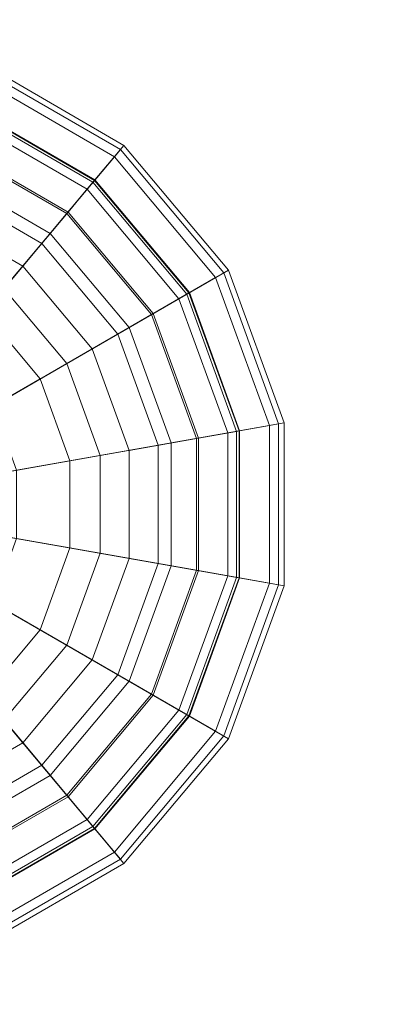
# Model space of a CAD drawing. Units: inches. Extents: x 375 to 1122, y 27 to 1069.
# Tile 93 of 155: x 730.25 to 731.282, y 859.033 to 861.878. Entities that reach past the tile are written whole.
import ezdxf

# ---------------------------------------------------------------- set-up
doc = ezdxf.new("R2010")
doc.units = ezdxf.units.IN
doc.layers.add('A-ANNO-DIMS', color=2, linetype='Continuous', lineweight=18)
doc.layers.add('Furniture', color=30, linetype='Continuous', lineweight=18)
doc.styles.get("Standard").update_dxf_attribs({"font": 'arial.ttf'})
doc.dimstyles.new('ISO-25', dxfattribs={"dimtxt": 12, "dimasz": 2.5, "dimexe": 1.5, "dimexo": 1.5, "dimtad": 1, "dimdec": 1, "dimlunit": 3, "dimtxsty": 'Standard', "dimblk": 'ARCHTICK', "dimcen": 2.5, "dimadec": 0, "dimazin": 0, "dimtfac": 1, "dimtdec": 1, "dimtmove": 0, "dimatfit": 3, "dimfxl": 1.5, "dimfxlon": 1, "dimarcsym": 0})

# ---------------------------------------------------------------- blocks, each defined once
blk = doc.blocks.new('A$C403C54AD')
for points in [[(1.940462, 1.15174, -0.060915), (1.946342, 1.118392, -0.057836), (1.946342, 1.118392, -0.057836), (1.929411, 1.147718, -0.060915)], [(1.941029, 1.148524, -0.057684), (1.940462, 1.15174, -0.060915), (1.929411, 1.147718, -0.060915), (1.931044, 1.144889, -0.057684)], [(1.941036, 1.148484, 0.102069), (1.940532, 1.151347, 0.088845), (1.929611, 1.147372, 0.088845), (1.931064, 1.144854, 0.102069)], [(1.940532, 1.151347, 0.088845), (1.940649, 1.150682, 0.060603), (1.929948, 1.146788, 0.060603), (1.929611, 1.147372, 0.088845)], [(1.952223, 1.15174, -0.060915), (1.946342, 1.118392, -0.057836), (1.946342, 1.118392, -0.057836), (1.940462, 1.15174, -0.060915)], [(1.951655, 1.148524, -0.057684), (1.952223, 1.15174, -0.060915), (1.940462, 1.15174, -0.060915), (1.941029, 1.148524, -0.057684)], [(1.951648, 1.148484, 0.102069), (1.952153, 1.151347, 0.088845), (1.940532, 1.151347, 0.088845), (1.941036, 1.148484, 0.102069)], [(1.952153, 1.151347, 0.088845), (1.952036, 1.150682, 0.060603), (1.940649, 1.150682, 0.060603), (1.940532, 1.151347, 0.088845)], [(1.963274, 1.147718, -0.060915), (1.946342, 1.118392, -0.057836), (1.946342, 1.118392, -0.057836), (1.952223, 1.15174, -0.060915)], [(1.96162, 1.144854, 0.102069), (1.963074, 1.147372, 0.088845), (1.952153, 1.151347, 0.088845), (1.951648, 1.148484, 0.102069)], [(1.961641, 1.144889, -0.057684), (1.963274, 1.147718, -0.060915), (1.952223, 1.15174, -0.060915), (1.951655, 1.148524, -0.057684)], [(1.963074, 1.147372, 0.088845), (1.962737, 1.146788, 0.060603), (1.952036, 1.150682, 0.060603), (1.952153, 1.151347, 0.088845)], [(1.940649, 1.150682, 0.060603), (1.94158, 1.145399, 0.042594), (1.932631, 1.142142, 0.042594), (1.929948, 1.146788, 0.060603)], [(1.952036, 1.150682, 0.060603), (1.951105, 1.145399, 0.042594), (1.94158, 1.145399, 0.042594), (1.940649, 1.150682, 0.060603)], [(1.962737, 1.146788, 0.060603), (1.960054, 1.142142, 0.042594), (1.951105, 1.145399, 0.042594), (1.952036, 1.150682, 0.060603)], [(1.943874, 1.13239, -0.054409), (1.941029, 1.148524, -0.057684), (1.931044, 1.144889, -0.057684), (1.939235, 1.130702, -0.054409)], [(1.941904, 1.143563, 0.111475), (1.941036, 1.148484, 0.102069), (1.931064, 1.144854, 0.102069), (1.933563, 1.140527, 0.111475)], [(1.941067, 1.148309, 0.088628), (1.941555, 1.145542, 0.101264), (1.932558, 1.142268, 0.101264), (1.931153, 1.144701, 0.088628)], [(1.941182, 1.147661, 0.061088), (1.941067, 1.148309, 0.088628), (1.931153, 1.144701, 0.088628), (1.931482, 1.144131, 0.061088)], [(1.948811, 1.13239, -0.054409), (1.951655, 1.148524, -0.057684), (1.941029, 1.148524, -0.057684), (1.943874, 1.13239, -0.054409)], [(1.950781, 1.143563, 0.111475), (1.951648, 1.148484, 0.102069), (1.941036, 1.148484, 0.102069), (1.941904, 1.143563, 0.111475)], [(1.951618, 1.148309, 0.088628), (1.95113, 1.145542, 0.101264), (1.941555, 1.145542, 0.101264), (1.941067, 1.148309, 0.088628)], [(1.951503, 1.147661, 0.061088), (1.951618, 1.148309, 0.088628), (1.941067, 1.148309, 0.088628), (1.941182, 1.147661, 0.061088)], [(1.95345, 1.130702, -0.054409), (1.961641, 1.144889, -0.057684), (1.951655, 1.148524, -0.057684), (1.948811, 1.13239, -0.054409)], [(1.959122, 1.140527, 0.111475), (1.96162, 1.144854, 0.102069), (1.951648, 1.148484, 0.102069), (1.950781, 1.143563, 0.111475)], [(1.961532, 1.144701, 0.088628), (1.960127, 1.142268, 0.101264), (1.95113, 1.145542, 0.101264), (1.951618, 1.148309, 0.088628)], [(1.961203, 1.144131, 0.061088), (1.961532, 1.144701, 0.088628), (1.951618, 1.148309, 0.088628), (1.951503, 1.147661, 0.061088)], [(1.929411, 1.147718, -0.060915), (1.946342, 1.118392, -0.057836), (1.946342, 1.118392, -0.057836), (1.920403, 1.140158, -0.060915)], [(1.931044, 1.144889, -0.057684), (1.929411, 1.147718, -0.060915), (1.920403, 1.140158, -0.060915), (1.922904, 1.138059, -0.057684)], [(1.942068, 1.142631, 0.043942), (1.941182, 1.147661, 0.061088), (1.931482, 1.144131, 0.061088), (1.934036, 1.139708, 0.043942)], [(1.950616, 1.142631, 0.043942), (1.951503, 1.147661, 0.061088), (1.941182, 1.147661, 0.061088), (1.942068, 1.142631, 0.043942)], [(1.972282, 1.140158, -0.060915), (1.946342, 1.118392, -0.057836), (1.946342, 1.118392, -0.057836), (1.963274, 1.147718, -0.060915)], [(1.958649, 1.139708, 0.043942), (1.961203, 1.144131, 0.061088), (1.951503, 1.147661, 0.061088), (1.950616, 1.142631, 0.043942)], [(1.969781, 1.138059, -0.057684), (1.972282, 1.140158, -0.060915), (1.963274, 1.147718, -0.060915), (1.961641, 1.144889, -0.057684)], [(1.931064, 1.144854, 0.102069), (1.929611, 1.147372, 0.088845), (1.920708, 1.139902, 0.088845), (1.922935, 1.138033, 0.102069)], [(1.929611, 1.147372, 0.088845), (1.929948, 1.146788, 0.060603), (1.921225, 1.139468, 0.060603), (1.920708, 1.139902, 0.088845)], [(1.96975, 1.138033, 0.102069), (1.971977, 1.139902, 0.088845), (1.963074, 1.147372, 0.088845), (1.96162, 1.144854, 0.102069)], [(1.971977, 1.139902, 0.088845), (1.97146, 1.139468, 0.060603), (1.962737, 1.146788, 0.060603), (1.963074, 1.147372, 0.088845)], [(1.929948, 1.146788, 0.060603), (1.932631, 1.142142, 0.042594), (1.925335, 1.13602, 0.042594), (1.921225, 1.139468, 0.060603)], [(1.97146, 1.139468, 0.060603), (1.96735, 1.13602, 0.042594), (1.960054, 1.142142, 0.042594), (1.962737, 1.146788, 0.060603)], [(1.941555, 1.145542, 0.101264), (1.942439, 1.140532, 0.111475), (1.935102, 1.137861, 0.111475), (1.932558, 1.142268, 0.101264)], [(1.94158, 1.145399, 0.042594), (1.942807, 1.13844, 0.032362), (1.936164, 1.136022, 0.032362), (1.932631, 1.142142, 0.042594)], [(1.95113, 1.145542, 0.101264), (1.950246, 1.140532, 0.111475), (1.942439, 1.140532, 0.111475), (1.941555, 1.145542, 0.101264)], [(1.951105, 1.145399, 0.042594), (1.949878, 1.13844, 0.032362), (1.942807, 1.13844, 0.032362), (1.94158, 1.145399, 0.042594)], [(1.960054, 1.142142, 0.042594), (1.956521, 1.136022, 0.032362), (1.949878, 1.13844, 0.032362), (1.951105, 1.145399, 0.042594)], [(1.960127, 1.142268, 0.101264), (1.957583, 1.137861, 0.111475), (1.950246, 1.140532, 0.111475), (1.95113, 1.145542, 0.101264)], [(1.939235, 1.130702, -0.054409), (1.931044, 1.144889, -0.057684), (1.922904, 1.138059, -0.057684), (1.935454, 1.127529, -0.054409)], [(1.933563, 1.140527, 0.111475), (1.931064, 1.144854, 0.102069), (1.922935, 1.138033, 0.102069), (1.926763, 1.134821, 0.111475)], [(1.931153, 1.144701, 0.088628), (1.932558, 1.142268, 0.101264), (1.925223, 1.136113, 0.101264), (1.923071, 1.137919, 0.088628)], [(1.931482, 1.144131, 0.061088), (1.931153, 1.144701, 0.088628), (1.923071, 1.137919, 0.088628), (1.923575, 1.137496, 0.061088)], [(1.957231, 1.127529, -0.054409), (1.969781, 1.138059, -0.057684), (1.961641, 1.144889, -0.057684), (1.95345, 1.130702, -0.054409)], [(1.965922, 1.134821, 0.111475), (1.96975, 1.138033, 0.102069), (1.96162, 1.144854, 0.102069), (1.959122, 1.140527, 0.111475)], [(1.969614, 1.137919, 0.088628), (1.967462, 1.136113, 0.101264), (1.960127, 1.142268, 0.101264), (1.961532, 1.144701, 0.088628)], [(1.96911, 1.137496, 0.061088), (1.969614, 1.137919, 0.088628), (1.961532, 1.144701, 0.088628), (1.961203, 1.144131, 0.061088)], [(1.934036, 1.139708, 0.043942), (1.931482, 1.144131, 0.061088), (1.923575, 1.137496, 0.061088), (1.927488, 1.134213, 0.043942)], [(1.965197, 1.134213, 0.043942), (1.96911, 1.137496, 0.061088), (1.961203, 1.144131, 0.061088), (1.958649, 1.139708, 0.043942)], [(1.942439, 1.140532, 0.111475), (1.941904, 1.143563, 0.111475), (1.933563, 1.140527, 0.111475), (1.935102, 1.137861, 0.111475)], [(1.950246, 1.140532, 0.111475), (1.950781, 1.143563, 0.111475), (1.941904, 1.143563, 0.111475), (1.942439, 1.140532, 0.111475)], [(1.957583, 1.137861, 0.111475), (1.959122, 1.140527, 0.111475), (1.950781, 1.143563, 0.111475), (1.950246, 1.140532, 0.111475)], [(1.943195, 1.136244, 0.03455), (1.942068, 1.142631, 0.043942), (1.934036, 1.139708, 0.043942), (1.937279, 1.134091, 0.03455)], [(1.94949, 1.136244, 0.03455), (1.950616, 1.142631, 0.043942), (1.942068, 1.142631, 0.043942), (1.943195, 1.136244, 0.03455)], [(1.955406, 1.134091, 0.03455), (1.958649, 1.139708, 0.043942), (1.950616, 1.142631, 0.043942), (1.94949, 1.136244, 0.03455)], [(1.932558, 1.142268, 0.101264), (1.935102, 1.137861, 0.111475), (1.929121, 1.132843, 0.111475), (1.925223, 1.136113, 0.101264)], [(1.932631, 1.142142, 0.042594), (1.936164, 1.136022, 0.032362), (1.930748, 1.131478, 0.032362), (1.925335, 1.13602, 0.042594)], [(1.96735, 1.13602, 0.042594), (1.961937, 1.131478, 0.032362), (1.956521, 1.136022, 0.032362), (1.960054, 1.142142, 0.042594)], [(1.967462, 1.136113, 0.101264), (1.963564, 1.132843, 0.111475), (1.957583, 1.137861, 0.111475), (1.960127, 1.142268, 0.101264)], [(1.935102, 1.137861, 0.111475), (1.933563, 1.140527, 0.111475), (1.926763, 1.134821, 0.111475), (1.929121, 1.132843, 0.111475)], [(1.963564, 1.132843, 0.111475), (1.965922, 1.134821, 0.111475), (1.959122, 1.140527, 0.111475), (1.957583, 1.137861, 0.111475)], [(1.920403, 1.140158, -0.060915), (1.946342, 1.118392, -0.057836), (1.946342, 1.118392, -0.057836), (1.914522, 1.129974, -0.060915)], [(1.922904, 1.138059, -0.057684), (1.920403, 1.140158, -0.060915), (1.914522, 1.129974, -0.060915), (1.917591, 1.128857, -0.057684)], [(1.922935, 1.138033, 0.102069), (1.920708, 1.139902, 0.088845), (1.914897, 1.129837, 0.088845), (1.917629, 1.128843, 0.102069)], [(1.920708, 1.139902, 0.088845), (1.921225, 1.139468, 0.060603), (1.915531, 1.129606, 0.060603), (1.914897, 1.129837, 0.088845)], [(1.937279, 1.134091, 0.03455), (1.934036, 1.139708, 0.043942), (1.927488, 1.134213, 0.043942), (1.932456, 1.130044, 0.03455)], [(1.978163, 1.129974, -0.060915), (1.946342, 1.118392, -0.057836), (1.946342, 1.118392, -0.057836), (1.972282, 1.140158, -0.060915)], [(1.960229, 1.130044, 0.03455), (1.965197, 1.134213, 0.043942), (1.958649, 1.139708, 0.043942), (1.955406, 1.134091, 0.03455)], [(1.975056, 1.128843, 0.102069), (1.977788, 1.129837, 0.088845), (1.971977, 1.139902, 0.088845), (1.96975, 1.138033, 0.102069)], [(1.975094, 1.128857, -0.057684), (1.978163, 1.129974, -0.060915), (1.972282, 1.140158, -0.060915), (1.969781, 1.138059, -0.057684)], [(1.977788, 1.129837, 0.088845), (1.977153, 1.129606, 0.060603), (1.97146, 1.139468, 0.060603), (1.971977, 1.139902, 0.088845)], [(1.921225, 1.139468, 0.060603), (1.925335, 1.13602, 0.042594), (1.920572, 1.127772, 0.042594), (1.915531, 1.129606, 0.060603)], [(1.977153, 1.129606, 0.060603), (1.972112, 1.127772, 0.042594), (1.96735, 1.13602, 0.042594), (1.97146, 1.139468, 0.060603)], [(1.942807, 1.13844, 0.032362), (1.944585, 1.128357, 0.024995), (1.941283, 1.127155, 0.024995), (1.936164, 1.136022, 0.032362)], [(1.949878, 1.13844, 0.032362), (1.9481, 1.128357, 0.024995), (1.944585, 1.128357, 0.024995), (1.942807, 1.13844, 0.032362)], [(1.956521, 1.136022, 0.032362), (1.951402, 1.127155, 0.024995), (1.9481, 1.128357, 0.024995), (1.949878, 1.13844, 0.032362)], [(1.935454, 1.127529, -0.054409), (1.922904, 1.138059, -0.057684), (1.917591, 1.128857, -0.057684), (1.932985, 1.123254, -0.054409)], [(1.926763, 1.134821, 0.111475), (1.922935, 1.138033, 0.102069), (1.917629, 1.128843, 0.102069), (1.922324, 1.127134, 0.111475)], [(1.923071, 1.137919, 0.088628), (1.925223, 1.136113, 0.101264), (1.920436, 1.127821, 0.101264), (1.917796, 1.128782, 0.088628)], [(1.923575, 1.137496, 0.061088), (1.923071, 1.137919, 0.088628), (1.917796, 1.128782, 0.088628), (1.918414, 1.128557, 0.061088)], [(1.9597, 1.123254, -0.054409), (1.975094, 1.128857, -0.057684), (1.969781, 1.138059, -0.057684), (1.957231, 1.127529, -0.054409)], [(1.970361, 1.127134, 0.111475), (1.975056, 1.128843, 0.102069), (1.96975, 1.138033, 0.102069), (1.965922, 1.134821, 0.111475)], [(1.974889, 1.128782, 0.088628), (1.972249, 1.127821, 0.101264), (1.967462, 1.136113, 0.101264), (1.969614, 1.137919, 0.088628)], [(1.974271, 1.128557, 0.061088), (1.974889, 1.128782, 0.088628), (1.969614, 1.137919, 0.088628), (1.96911, 1.137496, 0.061088)], [(1.927488, 1.134213, 0.043942), (1.923575, 1.137496, 0.061088), (1.918414, 1.128557, 0.061088), (1.923214, 1.12681, 0.043942)], [(1.969471, 1.12681, 0.043942), (1.974271, 1.128557, 0.061088), (1.96911, 1.137496, 0.061088), (1.965197, 1.134213, 0.043942)], [(1.944796, 1.127161, 0.027913), (1.943195, 1.136244, 0.03455), (1.937279, 1.134091, 0.03455), (1.94189, 1.126103, 0.027913)], [(1.947889, 1.127161, 0.027913), (1.94949, 1.136244, 0.03455), (1.943195, 1.136244, 0.03455), (1.944796, 1.127161, 0.027913)], [(1.950795, 1.126103, 0.027913), (1.955406, 1.134091, 0.03455), (1.94949, 1.136244, 0.03455), (1.947889, 1.127161, 0.027913)], [(1.925223, 1.136113, 0.101264), (1.929121, 1.132843, 0.111475), (1.925217, 1.126081, 0.111475), (1.920436, 1.127821, 0.101264)], [(1.925335, 1.13602, 0.042594), (1.930748, 1.131478, 0.032362), (1.927213, 1.125355, 0.032362), (1.920572, 1.127772, 0.042594)], [(1.936164, 1.136022, 0.032362), (1.941283, 1.127155, 0.024995), (1.938591, 1.124896, 0.024995), (1.930748, 1.131478, 0.032362)], [(1.961937, 1.131478, 0.032362), (1.954094, 1.124896, 0.024995), (1.951402, 1.127155, 0.024995), (1.956521, 1.136022, 0.032362)], [(1.972112, 1.127772, 0.042594), (1.965472, 1.125355, 0.032362), (1.961937, 1.131478, 0.032362), (1.96735, 1.13602, 0.042594)], [(1.972249, 1.127821, 0.101264), (1.967468, 1.126081, 0.111475), (1.963564, 1.132843, 0.111475), (1.967462, 1.136113, 0.101264)], [(1.929121, 1.132843, 0.111475), (1.926763, 1.134821, 0.111475), (1.922324, 1.127134, 0.111475), (1.925217, 1.126081, 0.111475)], [(1.967468, 1.126081, 0.111475), (1.970361, 1.127134, 0.111475), (1.965922, 1.134821, 0.111475), (1.963564, 1.132843, 0.111475)], [(1.932456, 1.130044, 0.03455), (1.927488, 1.134213, 0.043942), (1.923214, 1.12681, 0.043942), (1.929308, 1.124592, 0.03455)], [(1.94189, 1.126103, 0.027913), (1.937279, 1.134091, 0.03455), (1.932456, 1.130044, 0.03455), (1.939522, 1.124116, 0.027913)], [(1.953163, 1.124116, 0.027913), (1.960229, 1.130044, 0.03455), (1.955406, 1.134091, 0.03455), (1.950795, 1.126103, 0.027913)], [(1.963376, 1.124592, 0.03455), (1.969471, 1.12681, 0.043942), (1.965197, 1.134213, 0.043942), (1.960229, 1.130044, 0.03455)]]:
    blk.add_3dface(points)
blk = doc.blocks.new('_ArchTick')
at = {"color": 0, "linetype": 'ByBlock', "const_width": 0.15}
blk.add_lwpolyline([(-0.5, -0.5), (0.5, 0.5)], dxfattribs=at)
blk = doc.blocks.new('*D85')
at = {"layer": 'A-ANNO-DIMS', "color": 0, "lineweight": -2, "transparency": 16777216}
for p, q in [((401.5073, 868.5277), (398.5073, 868.5277)), ((400.0073, 814.5277), (400.0073, 868.5277)), ((401.5073, 814.5277), (398.5073, 814.5277))]:
    blk.add_line(p, q, dxfattribs=at)
at = {"layer": 'Defpoints', "color": 0, "transparency": 16777216}
for p in [(400.0073, 868.5277), (845.0073, 868.5277), (845.0073, 814.5277)]:
    blk.add_point(p, dxfattribs=at)
at = {"layer": 'A-ANNO-DIMS', "color": 0, "lineweight": -2, "transparency": 16777216, "xscale": 2.5, "yscale": 2.5, "zscale": 2.5}
for p, rotation in [((400.0073, 868.5277), 90), ((400.0073, 814.5277), 270)]:
    blk.add_blockref('_ArchTick', p, dxfattribs=dict(at, rotation=rotation))
at = {"layer": 'A-ANNO-DIMS', "color": 0, "transparency": 16777216, "insert": (393.2555, 841.5277), "char_height": 12, "attachment_point": 5, "rotation": 90}
blk.add_mtext('4\'-6"', dxfattribs=at)
blk = doc.blocks.new('*D88')
at = {"layer": 'A-ANNO-DIMS', "color": 0, "lineweight": -2, "transparency": 16777216}
for p, q in [((731.0073, 1052.5277), (731.0073, 1055.5277)), ((854.0073, 1052.5277), (854.0073, 1055.5277)), ((731.0073, 1054.0277), (854.0073, 1054.0277))]:
    blk.add_line(p, q, dxfattribs=at)
at = {"layer": 'Defpoints', "color": 0, "transparency": 16777216}
for p in [(854.0073, 1054.0277), (731.0073, 502.5277), (854.0073, 502.5277)]:
    blk.add_point(p, dxfattribs=at)
at = {"layer": 'A-ANNO-DIMS', "color": 0, "lineweight": -2, "transparency": 16777216, "xscale": 2.5, "yscale": 2.5, "zscale": 2.5, "rotation": 180}
blk.add_blockref('_ArchTick', (731.0073, 1054.0277), dxfattribs=at)
at = {"layer": 'A-ANNO-DIMS', "color": 0, "lineweight": -2, "transparency": 16777216, "xscale": 2.5, "yscale": 2.5, "zscale": 2.5}
blk.add_blockref('_ArchTick', (854.0073, 1054.0277), dxfattribs=at)
at = {"layer": 'A-ANNO-DIMS', "color": 0, "transparency": 16777216, "insert": (792.5073, 1060.7837), "char_height": 12, "attachment_point": 5}
blk.add_mtext('10\'-3"', dxfattribs=at)
blk = doc.blocks.new('*D91')
at = {"layer": 'A-ANNO-DIMS', "color": 0, "lineweight": -2, "transparency": 16777216}
for p, q in [((728.0073, 1052.5277), (728.0073, 1055.5277)), ((788.0073, 1052.5277), (788.0073, 1055.5277)), ((728.0073, 1054.0277), (788.0073, 1054.0277))]:
    blk.add_line(p, q, dxfattribs=at)
at = {"layer": 'Defpoints', "color": 0, "transparency": 16777216}
for p in [(788.0073, 1054.0277), (728.0073, 774.0277), (788.0073, 774.0277)]:
    blk.add_point(p, dxfattribs=at)
at = {"layer": 'A-ANNO-DIMS', "color": 0, "lineweight": -2, "transparency": 16777216, "xscale": 2.5, "yscale": 2.5, "zscale": 2.5, "rotation": 180}
blk.add_blockref('_ArchTick', (728.0073, 1054.0277), dxfattribs=at)
at = {"layer": 'A-ANNO-DIMS', "color": 0, "lineweight": -2, "transparency": 16777216, "xscale": 2.5, "yscale": 2.5, "zscale": 2.5}
blk.add_blockref('_ArchTick', (788.0073, 1054.0277), dxfattribs=at)
at = {"layer": 'A-ANNO-DIMS', "color": 0, "transparency": 16777216, "insert": (758.0073, 1060.7796), "char_height": 12, "attachment_point": 5}
blk.add_mtext('5\'-0"', dxfattribs=at)

msp = doc.modelspace()

# ---------------------------------------------------------------- block references
at = {"layer": 'Furniture', "xscale": 39.9918517141215, "yscale": 39.9918517141215, "zscale": 39.9918517141215, "rotation": 270}
msp.add_blockref('A$C403C54AD', (684.9549, 938.3156, 0.024), dxfattribs=at)

# ---------------------------------------------------------------- dimensions: what is measured, and where the dimension line sits
at = {"layer": 'A-ANNO-DIMS'}
for base, p1, p2, picture, middle in [((788.0073, 1054.0277), (728.0073, 774.0277), (788.0073, 774.0277), '*D91', (758.0073, 1060.7796)), ((854.0073, 1054.0277), (731.0073, 502.5277), (854.0073, 502.5277), '*D88', (792.5073, 1060.7837))]:
    dim = msp.add_linear_dim(base=base, p1=p1, p2=p2, dimstyle='ISO-25', override={"dimdec": 1, "dimlfac": 1, "dimrnd": 0, "dimzin": 1, "dimdsep": 46, "dimlunit": 4, "dimfrac": 2}, dxfattribs=at)
    dim.commit()
    dim.dimension.update_dxf_attribs({"geometry": picture, "text_midpoint": middle})
dim = msp.add_linear_dim(base=(400.0073, 868.5277), p1=(845.0073, 814.5277), p2=(845.0073, 868.5277), angle=90, dimstyle='ISO-25', override={"dimdec": 1, "dimlfac": 1, "dimrnd": 0, "dimzin": 1, "dimdsep": 46, "dimlunit": 4, "dimfrac": 2}, dxfattribs=at)
dim.commit()
dim.dimension.update_dxf_attribs({"geometry": '*D85', "text_midpoint": (393.2555, 841.5277)})

doc.saveas('drawing.dxf')
